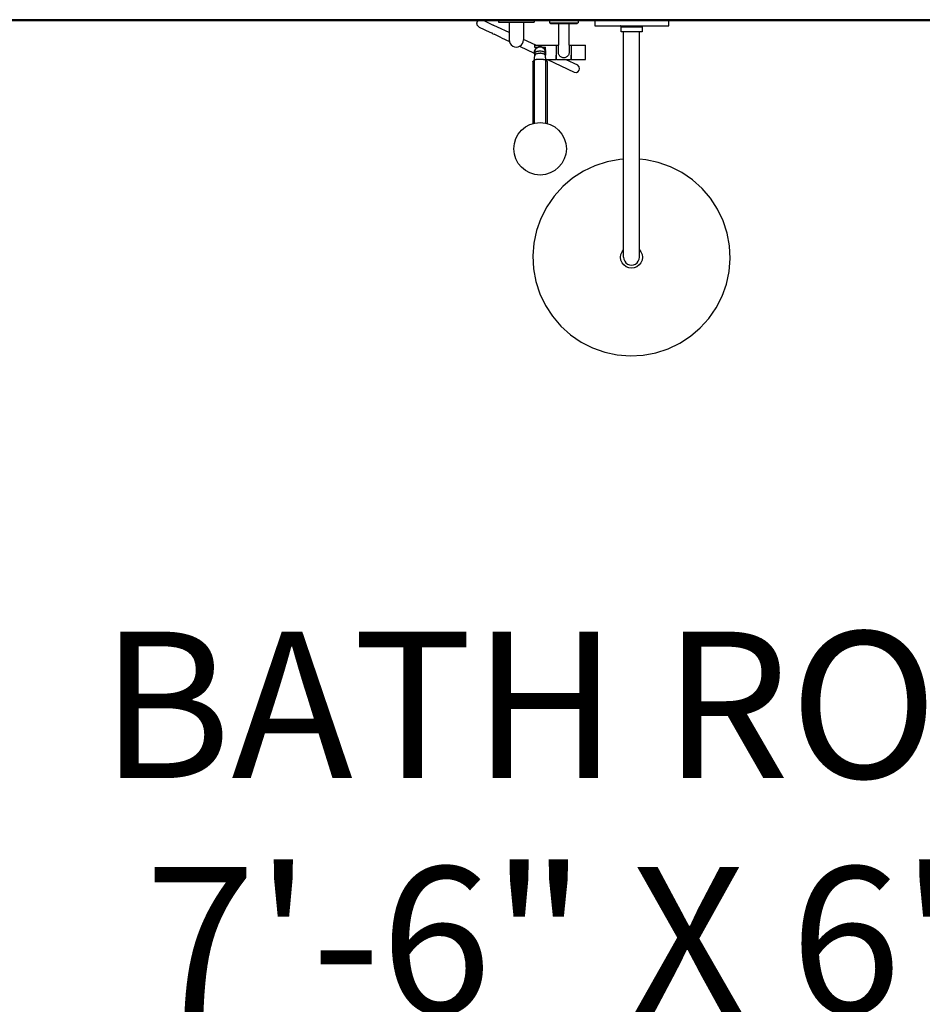
# Model space of a CAD drawing. Units: inches. Extents: x 64 to 1167, y 117 to 939.
# Tile 26 of 56: x 394 to 431, y 818 to 857. Entities that reach past the tile are written whole.
import ezdxf

# ---------------------------------------------------------------- set-up
doc = ezdxf.new("R2010")
doc.units = ezdxf.units.IN
doc.header["$MEASUREMENT"] = 0
for name, color, linetype, lineweight in [('A-ANNO-TEXT', 7, 'Continuous', 25), ('A-FLOR-FIXT', 8, 'Continuous', 18), ('A-WALL', 7, 'Continuous', 50)]:
    doc.layers.add(name, color=color, linetype=linetype, lineweight=lineweight)
doc.layers.add('Edges', color=7, linetype='Continuous')
doc.styles.get("Standard").update_dxf_attribs({"font": 'arial.ttf'})

# ---------------------------------------------------------------- blocks, each defined once
blk = doc.blocks.new('Handheld Shower set pl')
at = {"layer": 'Edges'}
for p, q in [((262, 340.8), (280.2, 332.2)), ((287.6, 328.7), (280.2, 332.2)), ((280.2, 332.2), (282.7, 331)), ((352.8, 340.8), (289.3, 340.8)), ((289.3, 340.8), (289.3, 337.7)), ((289.3, 337.7), (308.4, 337.7)), ((308.4, 337.7), (308.4, 318.8)), ((308.4, 337.7), (333.8, 337.7)), ((333.8, 337.7), (333.8, 306.8)), ((333.8, 337.7), (352.8, 337.7)), ((352.8, 340.8), (352.8, 337.7)), ((379.7, 340.5), (379.7, 336.5)), ((380.1, 340.7), (430.2, 340.7)), ((380.1, 336.2), (430.2, 336.2)), ((381.6, 335.3), (428.8, 335.3)), ((395.6, 335.3), (395.6, 296.4)), ((414.6, 296.4), (414.6, 335.3)), ((430.5, 340.5), (430.5, 336.5)), ((460.1, 340.8), (460.1, 330.7)), ((591.7, 340.8), (460.1, 340.8)), ((591.7, 330.7), (591.7, 340.8)), ((254.9, 328.7), (274.2, 319.6)), ((274.2, 319.6), (276.7, 318.4)), ((279.6, 317), (276.7, 318.4)), ((279.6, 317), (281.6, 316)), ((294.8, 309.8), (281.6, 316)), ((308.3, 318.9), (287.6, 328.7)), ((308.3, 318.9), (308.4, 318.8)), ((308.4, 318.8), (308.4, 305.9)), ((460.1, 330.7), (505.5, 330.7)), ((505.7, 330.7), (505.5, 330.7)), ((505.9, 330.6), (505.7, 330.7)), ((505.7, 330.7), (545.6, 330.7)), ((506.1, 330.5), (505.9, 330.6)), ((506.3, 330.4), (506.1, 330.5)), ((506.5, 330.3), (506.3, 330.4)), ((506.6, 330.1), (506.5, 330.3)), ((506.7, 329.9), (506.6, 330.1)), ((506.8, 329.7), (506.7, 329.9)), ((506.9, 329.5), (506.8, 329.7)), ((506.9, 329.3), (506.9, 329.5)), ((506.9, 329.1), (506.9, 329.3)), ((544.4, 329.1), (506.9, 329.1)), ((506.9, 320.4), (506.9, 328.9)), ((506.9, 328.9), (544.4, 328.9)), ((511.4, 320.4), (506.9, 320.4)), ((511.4, 94.2), (511.4, 320.4)), ((539.4, 320.4), (511.4, 320.4)), ((539.4, 94.2), (539.4, 320.4)), ((544.4, 320.4), (539.4, 320.4)), ((544.5, 329.5), (544.4, 329.3)), ((544.4, 329.3), (544.4, 329.1)), ((544.4, 328.9), (544.4, 320.4)), ((544.6, 329.9), (544.5, 329.7)), ((544.5, 329.7), (544.5, 329.5)), ((544.7, 330.1), (544.6, 329.9)), ((544.9, 330.3), (544.7, 330.1)), ((545, 330.4), (544.9, 330.3)), ((545.2, 330.5), (545, 330.4)), ((545.4, 330.6), (545.2, 330.5)), ((545.6, 330.7), (545.4, 330.6)), ((545.8, 330.7), (545.6, 330.7)), ((545.8, 330.7), (591.7, 330.7)), ((294.8, 309.8), (308.8, 303.2)), ((308.4, 305.9), (308.8, 303.2)), ((308.8, 303.2), (308.8, 302.6)), ((308.8, 302.6), (310.1, 299.6)), ((310.1, 299.6), (312.1, 296.9)), ((330.1, 296.9), (332.1, 299.6)), ((332.1, 299.6), (333.4, 302.6)), ((333.4, 302.6), (333.8, 305.9)), ((333.8, 306.8), (333.8, 305.9)), ((355.7, 296.4), (333.8, 306.8)), ((312.1, 296.9), (314.7, 294.9)), ((314.7, 294.9), (317.8, 293.7)), ((317.8, 293.7), (321.1, 293.2)), ((321.1, 293.2), (324.4, 293.7)), ((324.4, 293.7), (326.7, 294.6)), ((326.7, 294.6), (327.4, 294.9)), ((326.7, 294.6), (352.9, 282.2)), ((327.4, 294.9), (330.1, 296.9)), ((352.9, 285.6), (352.8, 284.3)), ((352.8, 284.3), (352.8, 283)), ((352.8, 283), (352.9, 282.2)), ((353.2, 286.9), (352.9, 285.6)), ((352.9, 282.2), (352.9, 281.8)), ((352.9, 281.8), (353.2, 280.5)), ((353.7, 288.1), (353.2, 286.9)), ((353.2, 280.5), (353.6, 279.7)), ((353.5, 296.4), (355.7, 296.4)), ((353.5, 296.4), (353.5, 293.2)), ((353.5, 293.2), (359.1, 293.2)), ((353.7, 285.5), (353.6, 284.3)), ((353.6, 283), (353.6, 284.3)), ((353.6, 283), (353.6, 282.5)), ((353.6, 282.5), (353.9, 283)), ((353.6, 283), (353.6, 281.9)), ((353.6, 282.1), (353.6, 282.5)), ((353.6, 281.9), (353.6, 282.1)), ((353.6, 282.1), (353.6, 281.3)), ((353.6, 281.3), (353.6, 281.9)), ((353.6, 279.7), (353.6, 281.9)), ((353.6, 279.7), (353.6, 279.5)), ((353.6, 278.6), (353.6, 279.7)), ((354.3, 289.2), (353.7, 288.1)), ((354, 286.6), (353.7, 285.5)), ((353.9, 283), (354.2, 283.5)), ((354.4, 287.8), (354, 286.6)), ((354, 279.6), (354.4, 280.1)), ((354.2, 283.5), (354.7, 284)), ((355.1, 290.3), (354.3, 289.2)), ((355, 288.8), (354.4, 287.8)), ((354.4, 280.1), (355, 280.5)), ((354.7, 284), (355.4, 284.5)), ((355.7, 289.8), (355, 288.8)), ((355, 280.5), (355.7, 280.9)), ((356, 291.2), (355.1, 290.3)), ((355.4, 284.5), (356.1, 284.9)), ((355.7, 296.4), (391.2, 296.4)), ((356.5, 290.6), (355.7, 289.8)), ((355.7, 280.9), (356.5, 281.3)), ((357, 292), (356, 291.2)), ((356.1, 284.9), (357, 285.3)), ((357.5, 291.4), (356.5, 290.6)), ((356.5, 281.3), (357.5, 281.6)), ((358.1, 292.7), (357, 292)), ((357, 285.3), (358, 285.7)), ((358.5, 292), (357.5, 291.4)), ((357.5, 281.6), (358.5, 281.9)), ((358, 285.7), (359, 285.9)), ((359.1, 293.2), (358.1, 292.7)), ((359.6, 292.6), (358.5, 292)), ((358.5, 281.9), (359.6, 282.1)), ((359, 285.9), (360.1, 286.2)), ((359.3, 293.3), (359.1, 293.2)), ((360.5, 293.7), (359.3, 293.3)), ((360.7, 292.9), (359.6, 292.6)), ((359.6, 282.1), (360.7, 282.3)), ((360.1, 286.2), (361.3, 286.3)), ((361.8, 293.9), (360.5, 293.7)), ((361.9, 293.1), (360.7, 292.9)), ((360.7, 282.3), (361.9, 282.4)), ((361.3, 286.3), (362.5, 286.4)), ((363.1, 294), (361.8, 293.9)), ((363.1, 293.2), (361.9, 293.1)), ((361.9, 282.4), (363.1, 282.4)), ((362.5, 286.4), (363.7, 286.4)), ((363.1, 292.9), (363.1, 297.1)), ((364.4, 293.9), (363.1, 294)), ((364.3, 293.1), (363.1, 293.2)), ((364.3, 282.4), (363.1, 282.4)), ((363.7, 286.4), (364.8, 286.3)), ((365.4, 292.9), (364.3, 293.1)), ((364.3, 282.4), (365.4, 282.3)), ((365.6, 293.7), (364.4, 293.9)), ((364.8, 286.3), (366, 286.2)), ((366.6, 292.6), (365.4, 292.9)), ((365.4, 282.3), (366.6, 282.1)), ((366.9, 293.3), (365.6, 293.7)), ((366, 286.2), (367.1, 285.9)), ((367.6, 292), (366.6, 292.6)), ((366.6, 282.1), (367.6, 281.9)), ((367, 293.2), (366.9, 293.3)), ((368, 292.7), (367, 293.2)), ((367, 293.2), (372.6, 293.2)), ((367.1, 285.9), (368.2, 285.7)), ((368.7, 291.4), (367.6, 292)), ((367.6, 281.9), (368.7, 281.6)), ((369.1, 292), (368, 292.7)), ((368.2, 285.7), (369.1, 285.3)), ((369.6, 290.6), (368.7, 291.4)), ((368.7, 281.6), (369.6, 281.3)), ((370.1, 291.2), (369.1, 292)), ((369.1, 285.3), (370, 284.9)), ((370.4, 289.8), (369.6, 290.6)), ((369.6, 281.3), (370.4, 280.9)), ((370, 284.9), (370.7, 284.5)), ((371, 290.3), (370.1, 291.2)), ((371.1, 288.8), (370.4, 289.8)), ((370.4, 280.9), (371.1, 280.5)), ((370.7, 284.5), (371.4, 284)), ((371.8, 289.2), (371, 290.3)), ((371.7, 287.8), (371.1, 288.8)), ((371.1, 280.5), (371.7, 280.1)), ((371.4, 284), (371.9, 283.5)), ((372.1, 286.6), (371.7, 287.8)), ((371.7, 280.1), (372.1, 279.6)), ((372.2, 288.5), (371.8, 289.2)), ((371.9, 283.5), (372.3, 283)), ((372.4, 285.5), (372.1, 286.6)), ((372.6, 288.3), (372.2, 288.5)), ((372.4, 288.1), (372.2, 288.5)), ((372.3, 283), (372.5, 282.5)), ((372.3, 281.3), (372.4, 281.9)), ((372.3, 280.7), (372.5, 281.3)), ((372.6, 287.7), (372.4, 288.1)), ((372.6, 284.3), (372.4, 285.5)), ((372.4, 281.9), (372.5, 282.3)), ((372.4, 279.3), (372.6, 279.7)), ((372.5, 282.5), (372.6, 283)), ((372.5, 282.5), (372.5, 282.3)), ((372.5, 282.1), (372.5, 282.3)), ((372.5, 282.1), (372.6, 281.9)), ((372.5, 282.1), (372.5, 281.3)), ((372.6, 281.9), (372.5, 281.3)), ((372.6, 288.3), (372.6, 293.2)), ((372.6, 288.3), (372.6, 287.7)), ((372.9, 286.9), (372.6, 287.7)), ((372.6, 283), (372.6, 284.3)), ((372.6, 283), (372.6, 281.9)), ((372.6, 281.9), (372.6, 279.7)), ((372.6, 279.7), (372.9, 280.5)), ((372.6, 279.7), (372.6, 278.6)), ((373.2, 285.6), (372.9, 286.9)), ((372.9, 280.5), (373.2, 281.8)), ((373.4, 284.3), (373.2, 285.6)), ((373.2, 281.8), (373.4, 283)), ((373.4, 283), (373.4, 284.3)), ((391.6, 296), (391.6, 271.4)), ((392, 295.6), (391.6, 295.6)), ((392, 295.6), (392, 279.3)), ((392, 295.6), (392, 279.1)), ((393.2, 296.4), (395.6, 296.4)), ((395.6, 283.7), (395.6, 296.4)), ((395.7, 282.5), (395.6, 283.7)), ((395.9, 281.3), (395.7, 282.5)), ((396.3, 280.2), (395.9, 281.3)), ((396.8, 279.1), (396.3, 280.2)), ((414, 280.2), (413.5, 279.1)), ((414.3, 281.3), (414, 280.2)), ((414.6, 282.5), (414.3, 281.3)), ((414.6, 296.4), (417, 296.4)), ((414.6, 296.4), (414.6, 283.7)), ((414.6, 283.7), (414.6, 282.5)), ((418.2, 295.6), (418.2, 279.3)), ((418.2, 295.6), (418.2, 279.1)), ((418.2, 295.6), (418.6, 295.6)), ((418.6, 296), (418.6, 271.4)), ((419, 296.4), (443.2, 296.4)), ((443.9, 272), (443.9, 295.4)), ((350.4, 266.9), (350.5, 267.6)), ((350.4, 266.9), (350.4, 157.5)), ((350.5, 267.6), (350.8, 268.3)), ((350.8, 268.3), (351.3, 269)), ((351.3, 269), (351.9, 269.7)), ((351.9, 269.7), (352.8, 270.3)), ((352.8, 270.3), (353.1, 270.5)), ((353.3, 270.7), (353.1, 270.6)), ((353.1, 270.5), (353.1, 270.6)), ((353.1, 263.2), (353.1, 270.5)), ((353.1, 158.2), (353.1, 263.2)), ((353.4, 270.7), (353.3, 270.7)), ((353.5, 270.7), (353.4, 270.7)), ((353.5, 274.2), (353.6, 278.1)), ((353.5, 271.2), (353.5, 274.2)), ((353.5, 274.2), (353.6, 274.2)), ((353.5, 271.2), (353.5, 271)), ((353.6, 271), (353.5, 271.2)), ((353.5, 271), (353.6, 271)), ((353.6, 270.8), (353.5, 270.7)), ((353.7, 279.1), (353.6, 278.6)), ((353.6, 278.6), (353.6, 278.1)), ((353.6, 278.1), (353.6, 277.9)), ((353.6, 270.8), (353.6, 271)), ((353.6, 270.8), (353.8, 270.9)), ((353.8, 270.9), (353.6, 270.8)), ((353.6, 270.8), (353.6, 270.8)), ((353.6, 270.8), (353.6, 270.8)), ((353.7, 279.1), (354, 279.6)), ((353.8, 270.8), (353.9, 270.9)), ((353.8, 270.9), (353.8, 270.8)), ((353.9, 270.9), (354.1, 270.9)), ((354.1, 270.9), (354.2, 271)), ((354.2, 271), (354.4, 271)), ((354.4, 271), (354.5, 271)), ((354.5, 271), (354.7, 271.1)), ((354.7, 271.1), (354.9, 271.1)), ((354.9, 271.1), (355.1, 271.1)), ((355.1, 271.1), (355.2, 271.2)), ((355.2, 271.2), (355.4, 271.2)), ((355.4, 271.2), (355.6, 271.2)), ((355.6, 271.2), (355.8, 271.2)), ((355.8, 271.2), (355.9, 271.2)), ((355.9, 271.2), (356.1, 271.3)), ((356.1, 271.3), (356.3, 271.3)), ((356.3, 271.3), (356.4, 271.3)), ((356.6, 271.3), (356.4, 271.3)), ((356.7, 271.3), (356.6, 271.3)), ((356.9, 271.3), (356.7, 271.3)), ((369.2, 271.3), (356.9, 271.3)), ((369.4, 271.3), (369.2, 271.3)), ((369.5, 271.3), (369.4, 271.3)), ((369.5, 271.3), (369.7, 271.3)), ((369.7, 271.3), (369.8, 271.3)), ((369.8, 271.3), (370, 271.3)), ((370, 271.3), (370.2, 271.2)), ((370.2, 271.2), (370.4, 271.2)), ((370.4, 271.2), (370.5, 271.2)), ((370.5, 271.2), (370.7, 271.2)), ((370.7, 271.2), (370.9, 271.2)), ((370.9, 271.2), (371.1, 271.1)), ((371.1, 271.1), (371.2, 271.1)), ((371.2, 271.1), (371.4, 271.1)), ((371.4, 271.1), (371.6, 271)), ((371.6, 271), (371.7, 271)), ((371.7, 271), (371.9, 271)), ((371.9, 271), (372.1, 270.9)), ((372.1, 279.6), (372.4, 279.2)), ((372.1, 270.9), (372.2, 270.9)), ((372.2, 270.9), (372.3, 270.8)), ((372.3, 277.4), (372.4, 277.6)), ((372.3, 274.2), (372.6, 274.2)), ((372.3, 271), (372.6, 271)), ((372.3, 270.9), (372.3, 270.8)), ((372.3, 270.9), (372.5, 270.8)), ((372.3, 270.8), (372.4, 270.8)), ((372.4, 279.2), (372.4, 279.3)), ((372.4, 279.1), (372.4, 279.2)), ((372.6, 278.6), (372.4, 279.1)), ((372.4, 277.6), (372.6, 278.1)), ((372.4, 270.8), (372.5, 270.8)), ((372.5, 270.8), (372.5, 270.8)), ((372.5, 270.8), (372.6, 270.8)), ((372.6, 278.1), (372.6, 278.6)), ((372.6, 274.2), (372.6, 278.1)), ((372.6, 274.2), (372.6, 271)), ((372.6, 271), (376.4, 271)), ((372.6, 271), (372.6, 270.8)), ((372.6, 270.8), (372.6, 270.7)), ((372.6, 270.7), (372.7, 270.7)), ((372.7, 270.7), (372.9, 270.7)), ((372.7, 270.7), (372.9, 270.6)), ((372.7, 270.7), (372.7, 270.7)), ((372.9, 270.7), (373, 270.6)), ((372.9, 270.7), (372.9, 270.6)), ((372.9, 270.6), (373, 270.5)), ((373, 270.6), (373, 270.5)), ((373, 270.5), (373, 158.3)), ((373, 270.5), (373.3, 270.3)), ((373.3, 270.3), (374.2, 269.7)), ((374.2, 269.7), (374.9, 269)), ((374.9, 269), (375.4, 268.3)), ((375.4, 268.3), (375.7, 267.6)), ((375.7, 267.6), (375.8, 266.9)), ((375.8, 266.9), (375.8, 157.6)), ((376.4, 271), (391.2, 271)), ((376.4, 271), (423.4, 248.7)), ((392, 271.8), (391.6, 271.8)), ((392, 279.3), (392, 279.1)), ((392, 279.3), (392, 279.1)), ((392, 279.1), (392, 278)), ((392, 279.1), (392, 278)), ((392, 279.1), (392, 279.1)), ((392, 279.1), (392, 279.1)), ((392, 271.8), (392, 279.1)), ((392, 271.8), (392, 278)), ((392, 271.8), (392, 271.8)), ((392, 271.8), (392.4, 271.8)), ((392, 271.8), (392.4, 271.8)), ((392.4, 271.8), (392.4, 271.8)), ((392.4, 271.7), (392.4, 271.8)), ((392.4, 271.6), (392.4, 271.7)), ((392.4, 271.7), (392.4, 271.7)), ((392.5, 271.6), (392.4, 271.6)), ((392.5, 271.5), (392.5, 271.6)), ((392.5, 271.5), (392.5, 271.5)), ((392.5, 271.4), (392.5, 271.5)), ((392.5, 271.4), (392.5, 271.4)), ((392.6, 271.3), (392.5, 271.4)), ((392.7, 271.2), (392.6, 271.3)), ((392.6, 271.3), (392.6, 271.3)), ((392.6, 271.3), (392.6, 271.3)), ((392.7, 271.2), (392.7, 271.2)), ((392.8, 271.2), (392.7, 271.2)), ((392.8, 271.1), (392.8, 271.2)), ((392.9, 271.1), (392.8, 271.1)), ((393, 271.1), (392.9, 271.1)), ((392.9, 271.1), (392.9, 271.1)), ((392.9, 271.1), (392.9, 271.1)), ((393, 271), (393, 271.1)), ((393, 271), (393.1, 271)), ((393.1, 271), (393.2, 271)), ((393.2, 271), (393.2, 271)), ((393.2, 271), (409, 271)), ((397.4, 278.1), (396.8, 279.1)), ((398.2, 277.2), (397.4, 278.1)), ((399, 276.4), (398.2, 277.2)), ((400, 275.7), (399, 276.4)), ((401.1, 275.1), (400, 275.7)), ((402.2, 274.6), (401.1, 275.1)), ((403.3, 274.3), (402.2, 274.6)), ((404.5, 274.2), (403.3, 274.3)), ((405.7, 274.2), (404.5, 274.2)), ((406.9, 274.3), (405.7, 274.2)), ((408.1, 274.6), (406.9, 274.3)), ((409.2, 275.1), (408.1, 274.6)), ((409, 271), (417, 271)), ((409, 271), (429.4, 261.4)), ((410.2, 275.7), (409.2, 275.1)), ((411.2, 276.4), (410.2, 275.7)), ((412.1, 277.2), (411.2, 276.4)), ((412.8, 278.1), (412.1, 277.2)), ((413.5, 279.1), (412.8, 278.1)), ((417.1, 271), (417, 271)), ((417.1, 271), (417.1, 271)), ((417.2, 271), (417.1, 271)), ((417.2, 271), (417.2, 271.1)), ((417.2, 271.1), (417.3, 271.1)), ((417.3, 271.1), (417.4, 271.1)), ((417.3, 271.1), (417.3, 271.1)), ((417.4, 271.1), (417.6, 271.3)), ((417.6, 271.3), (417.7, 271.4)), ((417.6, 271.3), (417.6, 271.3)), ((417.6, 271.3), (417.6, 271.3)), ((417.7, 271.5), (417.8, 271.6)), ((417.7, 271.5), (417.7, 271.5)), ((417.7, 271.4), (417.7, 271.5)), ((417.7, 271.4), (417.7, 271.4)), ((417.8, 271.8), (417.8, 271.8)), ((417.8, 271.7), (417.8, 271.8)), ((418.2, 271.8), (417.8, 271.8)), ((418.2, 271.8), (417.8, 271.8)), ((417.8, 271.6), (417.8, 271.7)), ((417.8, 271.7), (417.8, 271.7)), ((417.8, 271.6), (417.8, 271.6)), ((418.2, 271.8), (418.2, 279.1)), ((418.2, 271.8), (418.2, 278)), ((418.2, 271.8), (418.2, 271.8)), ((418.2, 271.8), (418.6, 271.8)), ((419, 271), (443.2, 271)), ((423.4, 248.7), (427.7, 248.2)), ((427.7, 248.2), (431, 249.9)), ((432.5, 258.3), (429.4, 261.4)), ((431, 249.9), (432.7, 252.1)), ((433.3, 254.7), (432.5, 258.3)), ((432.7, 252.1), (433.3, 254.7)), ((482.4, 89.7), (460.6, 82.7)), ((504.9, 93.9), (482.4, 89.7)), ((511.4, 94.2), (504.9, 93.9)), ((511.4, -66.4), (511.4, 94.2)), ((550.6, 93.3), (539.4, 94.2)), ((539.4, -66.4), (539.4, 94.2)), ((573, 88.5), (550.6, 93.3)), ((594.6, 80.9), (573, 88.5)), ((440, 72.8), (420.8, 60.4)), ((460.6, 82.7), (440, 72.8)), ((614.9, 70.5), (594.6, 80.9)), ((633.8, 57.5), (614.9, 70.5)), ((420.8, 60.4), (403.4, 45.5)), ((650.8, 42.2), (633.8, 57.5)), ((403.4, 45.5), (388, 28.5)), ((665.7, 24.8), (650.8, 42.2)), ((388, 28.5), (375.1, 9.6)), ((678.1, 5.6), (665.7, 24.8)), ((375.1, 9.6), (364.7, -10.8)), ((688, -15.1), (678.1, 5.6)), ((364.7, -10.8), (357, -32.3)), ((695, -36.9), (688, -15.1)), ((357, -32.3), (352.2, -54.7)), ((699.2, -59.4), (695, -36.9)), ((352.2, -54.7), (350.4, -77.5)), ((508.6, -70.1), (511.4, -66.4)), ((511.4, -79.8), (511.4, -66.4)), ((539.4, -66.4), (542.2, -70.1)), ((539.4, -79.8), (539.4, -66.4)), ((700.4, -82.3), (699.2, -59.4)), ((350.4, -77.5), (351.6, -100.4)), ((506, -79.8), (506.7, -74.8)), ((506.7, -84.8), (506, -79.8)), ((506.7, -74.8), (508.6, -70.1)), ((508.6, -89.5), (506.7, -84.8)), ((511.4, -79.8), (511.9, -83.4)), ((511.9, -83.4), (513.3, -86.8)), ((513.3, -86.8), (515.5, -89.7)), ((535.3, -89.7), (537.5, -86.8)), ((537.5, -86.8), (538.9, -83.4)), ((538.9, -83.4), (539.4, -79.8)), ((542.2, -70.1), (544.1, -74.8)), ((544.1, -84.8), (542.2, -89.5)), ((544.1, -74.8), (544.8, -79.8)), ((544.8, -79.8), (544.1, -84.8)), ((698.6, -105.1), (700.4, -82.3)), ((351.6, -100.4), (355.8, -122.9)), ((511.7, -93.5), (508.6, -89.5)), ((515.7, -96.6), (511.7, -93.5)), ((515.5, -89.7), (518.4, -91.9)), ((520.4, -98.5), (515.7, -96.6)), ((518.4, -91.9), (521.8, -93.3)), ((525.4, -99.2), (520.4, -98.5)), ((521.8, -93.3), (525.4, -93.8)), ((525.4, -93.8), (529, -93.3)), ((530.4, -98.5), (525.4, -99.2)), ((529, -93.3), (532.4, -91.9)), ((535.1, -96.6), (530.4, -98.5)), ((532.4, -91.9), (535.3, -89.7)), ((539.1, -93.5), (535.1, -96.6)), ((542.2, -89.5), (539.1, -93.5)), ((693.8, -127.5), (698.6, -105.1)), ((355.8, -122.9), (362.9, -144.7)), ((686.2, -149), (693.8, -127.5)), ((362.9, -144.7), (372.7, -165.3)), ((675.8, -169.4), (686.2, -149)), ((372.7, -165.3), (385.2, -184.6)), ((662.8, -188.3), (675.8, -169.4)), ((385.2, -184.6), (400, -202)), ((647.5, -205.3), (662.8, -188.3)), ((400, -202), (417, -217.3)), ((630.1, -220.2), (647.5, -205.3)), ((417, -217.3), (435.9, -230.3)), ((610.9, -232.6), (630.1, -220.2)), ((435.9, -230.3), (456.3, -240.7)), ((456.3, -240.7), (477.9, -248.3)), ((568.4, -249.5), (590.2, -242.5)), ((590.2, -242.5), (610.9, -232.6)), ((477.9, -248.3), (500.2, -253.1)), ((500.2, -253.1), (523.1, -254.9)), ((523.1, -254.9), (545.9, -253.7)), ((545.9, -253.7), (568.4, -249.5))]:
    blk.add_line(p, q, dxfattribs=at)
blk.add_lwpolyline([(254.9, 328.7), (253.9, 329.7), (253.1, 330.5), (252.5, 331), (252.2, 331.4), (251.9, 331.7), (251.8, 332), (251.7, 332.2), (251.6, 332.4), (251.6, 332.6), (251.5, 332.9), (251.4, 333.3), (251.4, 333.6), (251.3, 334), (251.3, 334.4), (251.2, 334.8), (251.2, 335.2), (251.2, 335.6), (251.2, 336), (251.3, 336.3), (251.4, 336.7), (251.4, 337), (251.6, 337.3), (251.7, 337.6), (251.8, 337.9), (252, 338.2), (252.1, 338.5), (252.3, 338.8), (252.5, 339.1), (252.7, 339.4), (253, 339.6), (253.3, 339.9), (253.6, 340.1), (253.9, 340.4), (254.2, 340.6), (254.5, 340.8), (254.9, 341), (255.2, 341.2), (255.5, 341.3), (255.8, 341.5), (256, 341.6), (256.2, 341.7), (256.4, 341.8), (256.5, 341.8), (256.6, 341.8), (256.8, 341.8), (257, 341.8), (257.3, 341.8), (257.7, 341.7), (258.1, 341.7), (258.6, 341.6), (259.2, 341.5), (259.8, 341.4), (260.4, 341.3), (261, 341.2), (261.6, 341), (262, 340.8)], dxfattribs=at)
blk.add_circle((363.2, 112.7), 46.6, dxfattribs=at)
for centre, radius, start, end in [((380, 340.3), 0.344, 86.4523, 162.0345), ((380, 336.6), 0.344, 197.9655, 273.5477), ((381.6, 336.4), 1.16, 189.8715, 268.521), ((428.8, 336.4), 1.16, 271.479, 350.1285), ((430.2, 340.3), 0.344, 17.9655, 93.5477), ((430.2, 336.6), 0.344, 266.4523, 342.0345), ((391.1, 295.9), 0.512, 11.477, 75.5526), ((393.6, 294.5), 1.97, 102.3058, 144.97), ((416.6, 294.5), 1.97, 35.03, 77.6942), ((419.1, 295.9), 0.512, 104.4474, 168.523), ((442.8, 295.4), 1.08, 2.6678, 69.8908), ((391.1, 271.5), 0.512, 284.4474, 348.523), ((419.1, 271.5), 0.512, 191.477, 255.5526), ((442.8, 272), 1.08, 290.1092, 357.3322)]:
    blk.add_arc(centre, radius, start, end, dxfattribs=at)

msp = doc.modelspace()

# ---------------------------------------------------------------- linework, layer by layer
at = {"layer": 'A-WALL'}
msp.add_line((467.107, 857.2), (377.107, 857.2), dxfattribs=at)

# ---------------------------------------------------------------- block references
at = {"layer": 'A-FLOR-FIXT', "xscale": 0.0226728872221849, "yscale": 0.0226728872221849, "zscale": 0.0226728872221849}
msp.add_blockref('Handheld Shower set pl', (407.104, 849.472), dxfattribs=at)

# ---------------------------------------------------------------- texts
at = {"layer": 'A-ANNO-TEXT'}
for s, height, p in [('BATH ROOM', 5.8926, (397.637, 826.701)), (' 7\'-6" X 6\'-0"', 5.89263, (397.637, 817.235))]:
    msp.add_text(s, height=height, dxfattribs=at).set_placement(p)

doc.saveas('drawing.dxf')
